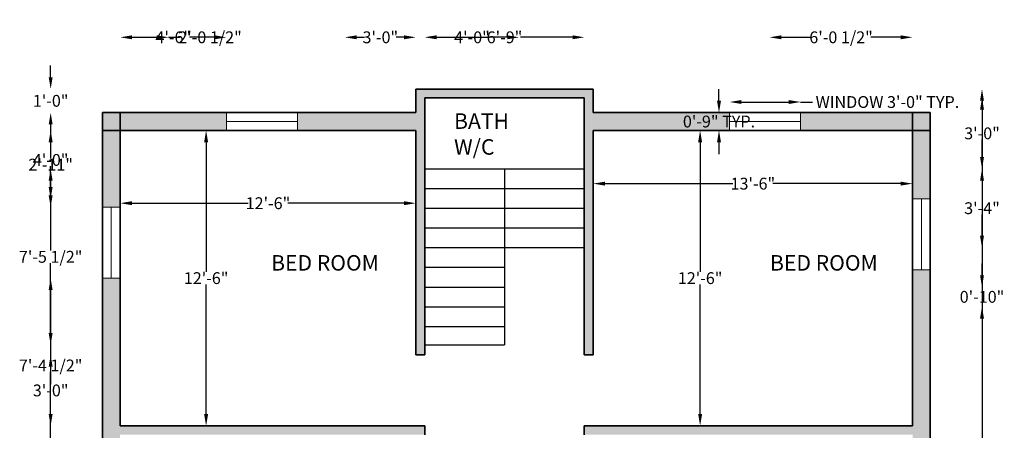
# Model space of a CAD drawing. Units: inches. Extents: x 759 to 1283, y 452 to 1038.
# Tile 3 of 3: x 780 to 1279, y 830 to 1038. Entities that reach past the tile are written whole.
import ezdxf

# ---------------------------------------------------------------- set-up
doc = ezdxf.new("R2010")
doc.units = ezdxf.units.IN
for name, color, linetype, lineweight in [('A-AREA-IDEN', 1, 'Continuous', 25), ('A-COLS', 7, 'Continuous', 35), ('A-COLS-PATT', 7, 'Continuous', 13), ('DIM', 2, 'Continuous', 18), ('STAIR', 7, 'Continuous', 25), ('WALL', 7, 'Continuous', 35), ('WINDOWS', 4, 'Continuous', 18)]:
    doc.layers.add(name, color=color, linetype=linetype, lineweight=lineweight)
doc.layers.add('A-WALL-PATT', color=67, linetype='Continuous', lineweight=13, true_color=0x727430)
doc.styles.get("Standard").update_dxf_attribs({"font": 'arial.ttf'})
doc.dimstyles.get("Standard").update_dxf_attribs({"dimtxt": 6, "dimasz": 6, "dimexe": 0.18, "dimexo": 0.0625, "dimgap": 0.09, "dimtad": 0, "dimtih": 1, "dimtoh": 1, "dimdec": 4, "dimzin": 0, "dimdsep": 46, "dimlunit": 4, "dimtxsty": 'Standard', "dimcen": 0.09, "dimse1": 1, "dimse2": 1, "dimadec": 0, "dimazin": 0, "dimtfac": 1, "dimtdec": 4, "dimtofl": 0, "dimtmove": 0, "dimatfit": 3, "dimfxl": 1, "dimtolj": 1, "dimtzin": 0, "dimarcsym": 0})

# ---------------------------------------------------------------- blocks, each defined once
blk = doc.blocks.new('*D1')
at = {"layer": 'Defpoints', "color": 0, "transparency": 16777216}
for p in [(830.47, 981.81), (980.47, 981.81), (980.47, 944.84)]:
    blk.add_point(p, dxfattribs=at)
at = {"layer": 'DIM', "color": 0, "lineweight": -2, "transparency": 16777216}
for p, q in [((836.47, 944.84), (895.35, 944.84)), ((974.47, 944.84), (915.58, 944.84))]:
    blk.add_line(p, q, dxfattribs=at)
at = {"layer": 'DIM', "color": 0, "transparency": 16777216}
for points in [[(836.47, 945.84), (836.47, 943.84), (830.47, 944.84)], [(974.47, 945.84), (974.47, 943.84), (980.47, 944.84)]]:
    blk.add_solid(points, dxfattribs=at)
at = {"layer": 'DIM', "color": 0, "transparency": 16777216, "insert": (905.47, 944.84), "char_height": 6, "attachment_point": 5}
blk.add_mtext('\\A1;12\'-6"', dxfattribs=at)
blk = doc.blocks.new('*D2')
at = {"layer": 'Defpoints', "color": 0, "transparency": 16777216}
for p in [(830.47, 981.81), (830.47, 831.81), (874.09, 831.81)]:
    blk.add_point(p, dxfattribs=at)
at = {"layer": 'DIM', "color": 0, "lineweight": -2, "transparency": 16777216}
for p, q in [((874.09, 975.81), (874.09, 909.96)), ((874.09, 837.81), (874.09, 903.65))]:
    blk.add_line(p, q, dxfattribs=at)
at = {"layer": 'DIM', "color": 0, "transparency": 16777216}
for points in [[(873.09, 975.81), (875.09, 975.81), (874.09, 981.81)], [(873.09, 837.81), (875.09, 837.81), (874.09, 831.81)]]:
    blk.add_solid(points, dxfattribs=at)
at = {"layer": 'DIM', "color": 0, "transparency": 16777216, "insert": (874.09, 906.81), "char_height": 6, "attachment_point": 5}
blk.add_mtext('\\A1;12\'-6"', dxfattribs=at)
blk = doc.blocks.new('*D3')
at = {"layer": 'Defpoints', "color": 0, "transparency": 16777216}
for p in [(1070.47, 981.81), (1232.47, 981.81), (1232.47, 954.77)]:
    blk.add_point(p, dxfattribs=at)
at = {"layer": 'DIM', "color": 0, "lineweight": -2, "transparency": 16777216}
for p, q in [((1076.47, 954.77), (1141.35, 954.77)), ((1226.47, 954.77), (1161.58, 954.77))]:
    blk.add_line(p, q, dxfattribs=at)
at = {"layer": 'DIM', "color": 0, "transparency": 16777216}
for points in [[(1076.47, 955.77), (1076.47, 953.77), (1070.47, 954.77)], [(1226.47, 955.77), (1226.47, 953.77), (1232.47, 954.77)]]:
    blk.add_solid(points, dxfattribs=at)
at = {"layer": 'DIM', "color": 0, "transparency": 16777216, "insert": (1151.47, 954.77), "char_height": 6, "attachment_point": 5}
blk.add_mtext('\\A1;13\'-6"', dxfattribs=at)
blk = doc.blocks.new('*D4')
at = {"layer": 'Defpoints', "color": 0, "transparency": 16777216}
for p in [(1232.47, 981.81), (1124.71, 831.81), (1232.47, 831.81)]:
    blk.add_point(p, dxfattribs=at)
at = {"layer": 'DIM', "color": 0, "lineweight": -2, "transparency": 16777216}
for p, q in [((1124.71, 975.81), (1124.71, 909.96)), ((1124.71, 837.81), (1124.71, 903.65))]:
    blk.add_line(p, q, dxfattribs=at)
at = {"layer": 'DIM', "color": 0, "transparency": 16777216}
for points in [[(1123.71, 975.81), (1125.71, 975.81), (1124.71, 981.81)], [(1123.71, 837.81), (1125.71, 837.81), (1124.71, 831.81)]]:
    blk.add_solid(points, dxfattribs=at)
at = {"layer": 'DIM', "color": 0, "transparency": 16777216, "insert": (1124.71, 906.81), "char_height": 6, "attachment_point": 5}
blk.add_mtext('\\A1;12\'-6"', dxfattribs=at)
blk = doc.blocks.new('WIN-36IN')
for p, q in [((0, 0), (0, 9)), ((0, 9), (36, 9)), ((36, 9), (36, 0)), ((0, 4.5), (36, 4.5)), ((36, 0), (0, 0))]:
    blk.add_line(p, q)
blk = doc.blocks.new('COL-9X9IN')
for p, q in [((0, 0), (0, 9)), ((0, 9), (9, 9)), ((9, 9), (9, 0)), ((9, 0), (0, 0))]:
    blk.add_line(p, q)
blk = doc.blocks.new('*D19')
at = {"layer": 'Defpoints', "color": 0, "transparency": 16777216}
for p in [(1175.68, 996.21), (1139.68, 990.81), (1175.68, 990.81)]:
    blk.add_point(p, dxfattribs=at)
at = {"layer": 'DIM', "color": 0, "lineweight": -2, "transparency": 16777216}
for p, q in [((1145.68, 996.21), (1169.68, 996.21)), ((1175.68, 996.21), (1181.68, 996.21))]:
    blk.add_line(p, q, dxfattribs=at)
at = {"layer": 'DIM', "color": 0, "transparency": 16777216}
for points in [[(1145.68, 997.21), (1145.68, 995.21), (1139.68, 996.21)], [(1169.68, 997.21), (1169.68, 995.21), (1175.68, 996.21)]]:
    blk.add_solid(points, dxfattribs=at)
at = {"layer": 'DIM', "color": 0, "transparency": 16777216, "insert": (1219.73, 996.21), "char_height": 6, "attachment_point": 5}
blk.add_mtext('\\A1;WINDOW 3\'-0" TYP.', dxfattribs=at)
blk = doc.blocks.new('*D20')
at = {"layer": 'Defpoints', "color": 0, "transparency": 16777216}
for p in [(1134.28, 990.81), (1139.68, 990.81), (1139.68, 981.81)]:
    blk.add_point(p, dxfattribs=at)
at = {"layer": 'DIM', "color": 0, "lineweight": -2, "transparency": 16777216}
for p, q in [((1134.28, 996.81), (1134.28, 1002.81)), ((1134.28, 975.81), (1134.28, 969.81))]:
    blk.add_line(p, q, dxfattribs=at)
at = {"layer": 'DIM', "color": 0, "transparency": 16777216}
for points in [[(1133.28, 996.81), (1135.28, 996.81), (1134.28, 990.81)], [(1133.28, 975.81), (1135.28, 975.81), (1134.28, 981.81)]]:
    blk.add_solid(points, dxfattribs=at)
at = {"layer": 'DIM', "color": 0, "transparency": 16777216, "insert": (1134.28, 986.31), "char_height": 6, "attachment_point": 5}
blk.add_mtext('\\A1;0\'-9" TYP.', dxfattribs=at)
blk = doc.blocks.new('*D24')
at = {"layer": 'Defpoints', "color": 0, "transparency": 16777216}
for p in [(1070.47, 1002.81), (1267.72, 1002.81), (1032.97, 486.81)]:
    blk.add_point(p, dxfattribs=at)
at = {"layer": 'DIM', "color": 0, "lineweight": -2, "transparency": 16777216}
for p, q in [((1267.72, 996.81), (1267.72, 747.96)), ((1267.72, 492.81), (1267.72, 741.65))]:
    blk.add_line(p, q, dxfattribs=at)
at = {"layer": 'DIM', "color": 0, "transparency": 16777216}
for points in [[(1266.72, 996.81), (1268.72, 996.81), (1267.72, 1002.81)], [(1266.72, 492.81), (1268.72, 492.81), (1267.72, 486.81)]]:
    blk.add_solid(points, dxfattribs=at)
at = {"layer": 'DIM', "color": 0, "transparency": 16777216, "insert": (1267.72, 744.81), "char_height": 6, "attachment_point": 5}
blk.add_mtext('\\A1;43\'-0"', dxfattribs=at)
blk = doc.blocks.new('*D25')
at = {"layer": 'Defpoints', "color": 0, "transparency": 16777216}
for p in [(1065.97, 1029.06), (984.97, 998.31), (1065.97, 998.31)]:
    blk.add_point(p, dxfattribs=at)
at = {"layer": 'DIM', "color": 0, "lineweight": -2, "transparency": 16777216}
for p, q in [((990.97, 1029.06), (1017.39, 1029.06)), ((1059.97, 1029.06), (1033.55, 1029.06))]:
    blk.add_line(p, q, dxfattribs=at)
at = {"layer": 'DIM', "color": 0, "transparency": 16777216}
for points in [[(990.97, 1030.06), (990.97, 1028.06), (984.97, 1029.06)], [(1059.97, 1030.06), (1059.97, 1028.06), (1065.97, 1029.06)]]:
    blk.add_solid(points, dxfattribs=at)
at = {"layer": 'DIM', "color": 0, "transparency": 16777216, "insert": (1025.47, 1029.06), "char_height": 6, "attachment_point": 5}
blk.add_mtext('\\A1;6\'-9"', dxfattribs=at)
blk = doc.blocks.new('*D26')
at = {"layer": 'Defpoints', "color": 0, "transparency": 16777216}
for p in [(795.216986, 1002.80698), (980.466986, 1002.80698), (980.466986, 990.80698)]:
    blk.add_point(p, dxfattribs=at)
at = {"layer": 'DIM', "color": 0, "lineweight": -2, "transparency": 16777216}
for p, q in [((795.216986, 1008.80698), (795.216986, 1014.80698)), ((795.216986, 984.80698), (795.216986, 978.80698))]:
    blk.add_line(p, q, dxfattribs=at)
at = {"layer": 'DIM', "color": 0, "transparency": 16777216}
for points in [[(794.216986, 1008.80698), (796.216986, 1008.80698), (795.216986, 1002.80698)], [(794.216986, 984.80698), (796.216986, 984.80698), (795.216986, 990.80698)]]:
    blk.add_solid(points, dxfattribs=at)
at = {"layer": 'DIM', "color": 0, "transparency": 16777216, "insert": (795.216986, 996.80698), "char_height": 6, "attachment_point": 5}
blk.add_mtext('\\A1;1\'-0"', dxfattribs=at)
blk = doc.blocks.new('*D27')
at = {"layer": 'Defpoints', "color": 0, "transparency": 16777216}
for p in [(1032.97, 1029.06), (984.97, 510.81), (1032.97, 510.81)]:
    blk.add_point(p, dxfattribs=at)
at = {"layer": 'DIM', "color": 0, "lineweight": -2, "transparency": 16777216}
for p, q in [((990.97, 1029.06), (1000.78, 1029.06)), ((1026.97, 1029.06), (1017.15, 1029.06))]:
    blk.add_line(p, q, dxfattribs=at)
at = {"layer": 'DIM', "color": 0, "transparency": 16777216}
for points in [[(990.97, 1030.06), (990.97, 1028.06), (984.97, 1029.06)], [(1026.97, 1030.06), (1026.97, 1028.06), (1032.97, 1029.06)]]:
    blk.add_solid(points, dxfattribs=at)
at = {"layer": 'DIM', "color": 0, "transparency": 16777216, "insert": (1008.97, 1029.06), "char_height": 6, "attachment_point": 5}
blk.add_mtext('\\A1;4\'-0"', dxfattribs=at)
blk = doc.blocks.new('*D29')
at = {"layer": 'Defpoints', "color": 0, "transparency": 16777216}
for p in [(830.47, 981.81), (884.41, 981.81), (884.41, 460.56)]:
    blk.add_point(p, dxfattribs=at)
at = {"layer": 'DIM', "color": 0, "lineweight": -2, "transparency": 16777216}
for p, q in [((836.47, 460.56), (849.25, 460.56)), ((878.41, 460.56), (865.62, 460.56))]:
    blk.add_line(p, q, dxfattribs=at)
at = {"layer": 'DIM', "color": 0, "transparency": 16777216}
for points in [[(836.47, 461.56), (836.47, 459.56), (830.47, 460.56)], [(878.41, 461.56), (878.41, 459.56), (884.41, 460.56)]]:
    blk.add_solid(points, dxfattribs=at)
at = {"layer": 'DIM', "color": 0, "transparency": 16777216, "insert": (857.44, 460.56), "char_height": 6, "attachment_point": 5}
blk.add_mtext('\\A1;4\'-6"', dxfattribs=at)
blk = doc.blocks.new('*D30')
at = {"layer": 'Defpoints', "color": 0, "transparency": 16777216}
for p in [(1175.68, 981.81), (1232.47, 981.81), (1232.47, 460.56)]:
    blk.add_point(p, dxfattribs=at)
at = {"layer": 'DIM', "color": 0, "lineweight": -2, "transparency": 16777216}
for p, q in [((1181.68, 460.56), (1195.89, 460.56)), ((1226.47, 460.56), (1212.26, 460.56))]:
    blk.add_line(p, q, dxfattribs=at)
at = {"layer": 'DIM', "color": 0, "transparency": 16777216}
for points in [[(1181.68, 461.56), (1181.68, 459.56), (1175.68, 460.56)], [(1226.47, 461.56), (1226.47, 459.56), (1232.47, 460.56)]]:
    blk.add_solid(points, dxfattribs=at)
at = {"layer": 'DIM', "color": 0, "transparency": 16777216, "insert": (1204.07, 460.56), "char_height": 6, "attachment_point": 5}
blk.add_mtext('\\A1;4\'-9"', dxfattribs=at)
blk = doc.blocks.new('*D31')
at = {"layer": 'Defpoints', "color": 0, "transparency": 16777216}
for p in [(884.41, 1029.06), (830.47, 519.81), (884.41, 519.81)]:
    blk.add_point(p, dxfattribs=at)
at = {"layer": 'DIM', "color": 0, "lineweight": -2, "transparency": 16777216}
for p, q in [((836.47, 1029.06), (849.25, 1029.06)), ((878.41, 1029.06), (865.62, 1029.06))]:
    blk.add_line(p, q, dxfattribs=at)
at = {"layer": 'DIM', "color": 0, "transparency": 16777216}
for points in [[(836.47, 1030.06), (836.47, 1028.06), (830.47, 1029.06)], [(878.41, 1030.06), (878.41, 1028.06), (884.41, 1029.06)]]:
    blk.add_solid(points, dxfattribs=at)
at = {"layer": 'DIM', "color": 0, "transparency": 16777216, "insert": (857.44, 1029.06), "char_height": 6, "attachment_point": 5}
blk.add_mtext('\\A1;4\'-6"', dxfattribs=at)
blk = doc.blocks.new('*D32')
at = {"layer": 'Defpoints', "color": 0, "transparency": 16777216}
for p in [(1232.47, 1029.06), (1159.97, 519.81), (1232.47, 519.81)]:
    blk.add_point(p, dxfattribs=at)
at = {"layer": 'DIM', "color": 0, "lineweight": -2, "transparency": 16777216}
for p, q in [((1165.97, 1029.06), (1181.15, 1029.06)), ((1226.47, 1029.06), (1211.29, 1029.06))]:
    blk.add_line(p, q, dxfattribs=at)
at = {"layer": 'DIM', "color": 0, "transparency": 16777216}
for points in [[(1165.97, 1030.06), (1165.97, 1028.06), (1159.97, 1029.06)], [(1226.47, 1030.06), (1226.47, 1028.06), (1232.47, 1029.06)]]:
    blk.add_solid(points, dxfattribs=at)
at = {"layer": 'DIM', "color": 0, "transparency": 16777216, "insert": (1196.22, 1029.06), "char_height": 6, "attachment_point": 5}
blk.add_mtext('\\A1;6\'-0 1/2"', dxfattribs=at)
blk = doc.blocks.new('*D33')
at = {"layer": 'Defpoints', "color": 0, "transparency": 16777216}
for p in [(821.47, 990.81), (795.22, 942.81), (821.47, 942.81)]:
    blk.add_point(p, dxfattribs=at)
at = {"layer": 'DIM', "color": 0, "lineweight": -2, "transparency": 16777216}
for p, q in [((795.22, 984.81), (795.22, 969.96)), ((795.22, 948.81), (795.22, 963.65))]:
    blk.add_line(p, q, dxfattribs=at)
at = {"layer": 'DIM', "color": 0, "transparency": 16777216}
for points in [[(794.22, 984.81), (796.22, 984.81), (795.22, 990.81)], [(794.22, 948.81), (796.22, 948.81), (795.22, 942.81)]]:
    blk.add_solid(points, dxfattribs=at)
at = {"layer": 'DIM', "color": 0, "transparency": 16777216, "insert": (795.22, 966.81), "char_height": 6, "attachment_point": 5}
blk.add_mtext('\\A1;4\'-0"', dxfattribs=at)
blk = doc.blocks.new('*D34')
at = {"layer": 'Defpoints', "color": 0, "transparency": 16777216}
for p in [(821.47, 906.81), (795.22, 818.14), (821.47, 818.14)]:
    blk.add_point(p, dxfattribs=at)
at = {"layer": 'DIM', "color": 0, "lineweight": -2, "transparency": 16777216}
for p, q in [((795.22, 900.81), (795.22, 865.67)), ((795.22, 824.14), (795.22, 859.28))]:
    blk.add_line(p, q, dxfattribs=at)
at = {"layer": 'DIM', "color": 0, "transparency": 16777216}
for points in [[(794.22, 900.81), (796.22, 900.81), (795.22, 906.81)], [(794.22, 824.14), (796.22, 824.14), (795.22, 818.14)]]:
    blk.add_solid(points, dxfattribs=at)
at = {"layer": 'DIM', "color": 0, "transparency": 16777216, "insert": (795.22, 862.47), "char_height": 6, "attachment_point": 5}
blk.add_mtext('\\A1;7\'-4 1/2"', dxfattribs=at)
blk = doc.blocks.new('*D37')
at = {"layer": 'Defpoints', "color": 0, "transparency": 16777216}
for p in [(1232.47, 981.81), (795.22, 947.03), (1232.47, 947.03)]:
    blk.add_point(p, dxfattribs=at)
at = {"layer": 'DIM', "color": 0, "lineweight": -2, "transparency": 16777216}
for p, q in [((795.22, 975.81), (795.22, 967.52)), ((795.22, 953.03), (795.22, 961.32))]:
    blk.add_line(p, q, dxfattribs=at)
at = {"layer": 'DIM', "color": 0, "transparency": 16777216}
for points in [[(794.22, 975.81), (796.22, 975.81), (795.22, 981.81)], [(794.22, 953.03), (796.22, 953.03), (795.22, 947.03)]]:
    blk.add_solid(points, dxfattribs=at)
at = {"layer": 'DIM', "color": 0, "transparency": 16777216, "insert": (795.22, 964.42), "char_height": 6, "attachment_point": 5}
blk.add_mtext('\\A1;2\'-11"', dxfattribs=at)
blk = doc.blocks.new('*D40')
at = {"layer": 'Defpoints', "color": 0, "transparency": 16777216}
for p in [(984.97, 998.31), (984.97, 962.31), (1267.72, 962.31)]:
    blk.add_point(p, dxfattribs=at)
at = {"layer": 'DIM', "color": 0, "lineweight": -2, "transparency": 16777216}
for p, q in [((1267.72, 992.31), (1267.72, 983.46)), ((1267.72, 968.31), (1267.72, 977.15))]:
    blk.add_line(p, q, dxfattribs=at)
at = {"layer": 'DIM', "color": 0, "transparency": 16777216}
for points in [[(1266.72, 992.31), (1268.72, 992.31), (1267.72, 998.31)], [(1266.72, 968.31), (1268.72, 968.31), (1267.72, 962.31)]]:
    blk.add_solid(points, dxfattribs=at)
at = {"layer": 'DIM', "color": 0, "transparency": 16777216, "insert": (1267.72, 980.31), "char_height": 6, "attachment_point": 5}
blk.add_mtext('\\A1;3\'-0"', dxfattribs=at)
blk = doc.blocks.new('*D41')
at = {"layer": 'Defpoints', "color": 0, "transparency": 16777216}
for p in [(984.966986, 872.954802), (1025.466986, 872.954802), (1025.466986, 460.55698)]:
    blk.add_point(p, dxfattribs=at)
at = {"layer": 'DIM', "color": 0, "lineweight": -2, "transparency": 16777216}
for p, q in [((978.966986, 460.55698), (972.966986, 460.55698)), ((1031.466986, 460.55698), (1037.466986, 460.55698))]:
    blk.add_line(p, q, dxfattribs=at)
at = {"layer": 'DIM', "color": 0, "transparency": 16777216}
for points in [[(978.966986, 461.55698), (978.966986, 459.55698), (984.966986, 460.55698)], [(1031.466986, 461.55698), (1031.466986, 459.55698), (1025.466986, 460.55698)]]:
    blk.add_solid(points, dxfattribs=at)
at = {"layer": 'DIM', "color": 0, "transparency": 16777216, "insert": (1005.216986, 460.55698), "char_height": 6, "attachment_point": 5}
blk.add_mtext('\\A1;3\'-4 1/2"', dxfattribs=at)
blk = doc.blocks.new('*D42')
at = {"layer": 'Defpoints', "color": 0, "transparency": 16777216}
for p in [(984.97, 867.81), (795.22, 831.81), (984.97, 831.81)]:
    blk.add_point(p, dxfattribs=at)
at = {"layer": 'DIM', "color": 0, "lineweight": -2, "transparency": 16777216}
for p, q in [((795.22, 861.81), (795.22, 852.96)), ((795.22, 837.81), (795.22, 846.65))]:
    blk.add_line(p, q, dxfattribs=at)
at = {"layer": 'DIM', "color": 0, "transparency": 16777216}
for points in [[(794.22, 861.81), (796.22, 861.81), (795.22, 867.81)], [(794.22, 837.81), (796.22, 837.81), (795.22, 831.81)]]:
    blk.add_solid(points, dxfattribs=at)
at = {"layer": 'DIM', "color": 0, "transparency": 16777216, "insert": (795.22, 849.81), "char_height": 6, "attachment_point": 5}
blk.add_mtext('\\A1;3\'-0"', dxfattribs=at)
blk = doc.blocks.new('*D46')
at = {"layer": 'Defpoints', "color": 0, "transparency": 16777216}
for p in [(980.47, 1029.06), (944.47, 660.31), (980.47, 660.31)]:
    blk.add_point(p, dxfattribs=at)
at = {"layer": 'DIM', "color": 0, "lineweight": -2, "transparency": 16777216}
for p, q in [((950.47, 1029.06), (954.4, 1029.06)), ((974.47, 1029.06), (970.53, 1029.06))]:
    blk.add_line(p, q, dxfattribs=at)
at = {"layer": 'DIM', "color": 0, "transparency": 16777216}
for points in [[(950.47, 1030.06), (950.47, 1028.06), (944.47, 1029.06)], [(974.47, 1030.06), (974.47, 1028.06), (980.47, 1029.06)]]:
    blk.add_solid(points, dxfattribs=at)
at = {"layer": 'DIM', "color": 0, "transparency": 16777216, "insert": (962.47, 1029.06), "char_height": 6, "attachment_point": 5}
blk.add_mtext('\\A1;3\'-0"', dxfattribs=at)
blk = doc.blocks.new('*D47')
at = {"layer": 'Defpoints', "color": 0, "transparency": 16777216}
for p in [(795.22, 962.31), (984.97, 962.31), (984.97, 872.95)]:
    blk.add_point(p, dxfattribs=at)
at = {"layer": 'DIM', "color": 0, "lineweight": -2, "transparency": 16777216}
for p, q in [((795.22, 956.31), (795.22, 920.82)), ((795.22, 878.95), (795.22, 914.44))]:
    blk.add_line(p, q, dxfattribs=at)
at = {"layer": 'DIM', "color": 0, "transparency": 16777216}
for points in [[(794.22, 956.31), (796.22, 956.31), (795.22, 962.31)], [(794.22, 878.95), (796.22, 878.95), (795.22, 872.95)]]:
    blk.add_solid(points, dxfattribs=at)
at = {"layer": 'DIM', "color": 0, "transparency": 16777216, "insert": (795.22, 917.63), "char_height": 6, "attachment_point": 5}
blk.add_mtext('\\A1;7\'-5 1/2"', dxfattribs=at)
blk = doc.blocks.new('*D48')
at = {"layer": 'Defpoints', "color": 0, "transparency": 16777216}
for p in [(1025.466986, 902.30698), (1267.716986, 902.30698), (1025.466986, 892.30698)]:
    blk.add_point(p, dxfattribs=at)
at = {"layer": 'DIM', "color": 0, "lineweight": -2, "transparency": 16777216}
for p, q in [((1267.716986, 908.30698), (1267.716986, 914.30698)), ((1267.716986, 886.30698), (1267.716986, 880.30698))]:
    blk.add_line(p, q, dxfattribs=at)
at = {"layer": 'DIM', "color": 0, "transparency": 16777216}
for points in [[(1266.716986, 908.30698), (1268.716986, 908.30698), (1267.716986, 902.30698)], [(1266.716986, 886.30698), (1268.716986, 886.30698), (1267.716986, 892.30698)]]:
    blk.add_solid(points, dxfattribs=at)
at = {"layer": 'DIM', "color": 0, "transparency": 16777216, "insert": (1267.716986, 897.30698), "char_height": 6, "attachment_point": 5}
blk.add_mtext('\\A1;0\'-10"', dxfattribs=at)
blk = doc.blocks.new('*D49')
at = {"layer": 'Defpoints', "color": 0, "transparency": 16777216}
for p in [(1065.97, 962.31), (1267.72, 962.31), (1065.97, 922.31)]:
    blk.add_point(p, dxfattribs=at)
at = {"layer": 'DIM', "color": 0, "lineweight": -2, "transparency": 16777216}
for p, q in [((1267.72, 956.31), (1267.72, 945.46)), ((1267.72, 928.31), (1267.72, 939.15))]:
    blk.add_line(p, q, dxfattribs=at)
at = {"layer": 'DIM', "color": 0, "transparency": 16777216}
for points in [[(1266.72, 956.31), (1268.72, 956.31), (1267.72, 962.31)], [(1266.72, 928.31), (1268.72, 928.31), (1267.72, 922.31)]]:
    blk.add_solid(points, dxfattribs=at)
at = {"layer": 'DIM', "color": 0, "transparency": 16777216, "insert": (1267.72, 942.31), "char_height": 6, "attachment_point": 5}
blk.add_mtext('\\A1;3\'-4"', dxfattribs=at)
blk = doc.blocks.new('*D50')
at = {"layer": 'Defpoints', "color": 0, "transparency": 16777216}
for p in [(854.96, 1029.06), (830.47, 664.81), (854.96, 664.81)]:
    blk.add_point(p, dxfattribs=at)
at = {"layer": 'DIM', "color": 0, "lineweight": -2, "transparency": 16777216}
for p, q in [((836.47, 1029.06), (848.96, 1029.06)), ((854.96, 1029.06), (860.96, 1029.06))]:
    blk.add_line(p, q, dxfattribs=at)
at = {"layer": 'DIM', "color": 0, "transparency": 16777216}
for points in [[(836.47, 1030.06), (836.47, 1028.06), (830.47, 1029.06)], [(848.96, 1030.06), (848.96, 1028.06), (854.96, 1029.06)]]:
    blk.add_solid(points, dxfattribs=at)
at = {"layer": 'DIM', "color": 0, "transparency": 16777216, "insert": (876.07, 1029.06), "char_height": 6, "attachment_point": 5}
blk.add_mtext('\\A1;2\'-0 1/2"', dxfattribs=at)

msp = doc.modelspace()

# ---------------------------------------------------------------- hatches: boundary and pattern name
at = {"layer": 'A-COLS-PATT'}
h = msp.add_hatch(color=256, dxfattribs=at)
h.dxf.hatch_style = 1
h.paths.add_polyline_path([(1241.46699, 990.80698), (1232.46699, 990.80698), (1232.46699, 981.80698), (1241.46699, 981.80698)])
h.paths.add_polyline_path([(830.46699, 990.80698), (821.46699, 990.80698), (821.46699, 981.80698), (830.46699, 981.80698)])
h.paths.add_polyline_path([(830.46699, 519.80698), (821.46699, 519.80698), (821.46699, 510.80698), (830.46699, 510.80698)])
h.paths.add_polyline_path([(1241.46699, 519.80698), (1232.46699, 519.80698), (1232.46699, 510.80698), (1241.46699, 510.80698)])
at = {"layer": 'A-WALL-PATT'}
h = msp.add_hatch(color=256, dxfattribs=at)
h.dxf.hatch_style = 1
h.paths.add_polyline_path([(1232.46699, 519.80698), (1159.97269, 519.80698), (1159.97269, 510.80698), (1232.46699, 510.80698)])
h.paths.add_polyline_path([(1241.46699, 580.365), (1232.46699, 580.365), (1232.46699, 519.80698), (1241.46699, 519.80698)])
h.paths.add_polyline_path([(1123.97269, 519.80698), (1032.96699, 519.80698), (1032.96699, 510.80698), (1123.97269, 510.80698)])
h.paths.add_polyline_path([(984.96699, 519.80698), (984.96699, 664.80698), (980.46699, 664.80698), (980.46699, 660.30698), (980.46699, 519.80698), (920.40841, 519.80698), (920.40841, 510.80698), (984.96699, 510.80698)])
h.paths.add_polyline_path([(884.40841, 519.80698), (830.46699, 519.80698), (830.46699, 510.80698), (884.40841, 510.80698)])
h.paths.add_polyline_path([(830.46699, 590.05698), (821.46699, 590.05698), (821.46699, 519.80698), (830.46699, 519.80698)])
h.paths.add_polyline_path([(830.46699, 660.30698), (944.46699, 660.30698), (944.46699, 664.80698), (830.46699, 664.80698), (830.46699, 691.13164), (821.46699, 691.13164), (821.46699, 626.05698), (830.46699, 626.05698)])
h.paths.add_polyline_path([(830.46699, 767.80698), (914.46699, 767.80698), (914.46699, 726.32345), (918.96699, 726.32345), (918.96699, 775.80521), (918.96699, 790.30698), (914.46699, 790.30698), (914.46699, 772.30698), (830.46699, 772.30698), (830.46699, 782.14186), (821.46699, 782.14186), (821.46699, 727.13164), (830.46699, 727.13164)])
h.paths.add_polyline_path([(830.46699, 906.80698), (821.46699, 906.80698), (821.46699, 818.14186), (830.46699, 818.14186), (830.46699, 827.30698), (984.96699, 827.30698), (984.96699, 831.80698), (980.46699, 831.80698), (830.46699, 831.80698)])
h.paths.add_polyline_path([(830.46699, 981.80698), (821.46699, 981.80698), (821.46699, 942.80698), (830.46699, 942.80698)])
h.paths.add_polyline_path([(884.40841, 990.80698), (830.46699, 990.80698), (830.46699, 981.80698), (884.40841, 981.80698)])
h.paths.add_polyline_path([(984.96699, 998.30698), (1065.96699, 998.30698), (1065.96699, 981.80698), (1065.96699, 867.80698), (1070.46699, 867.80698), (1070.46699, 981.80698), (1139.68016, 981.80698), (1139.68016, 990.80698), (1070.46699, 990.80698), (1070.46699, 1002.80698), (980.46699, 1002.80698), (980.46699, 990.80698), (920.40841, 990.80698), (920.40841, 981.80698), (980.46699, 981.80698), (980.46699, 867.80698), (984.96699, 867.80698), (984.96699, 981.80698)])
h.paths.add_polyline_path([(1232.46699, 990.80698), (1175.68016, 990.80698), (1175.68016, 981.80698), (1232.46699, 981.80698)])
h.paths.add_polyline_path([(1241.46699, 981.80698), (1232.46699, 981.80698), (1232.46699, 947.03418), (1241.46699, 947.03418)])
h.paths.add_polyline_path([(1241.46699, 911.03418), (1232.46699, 911.03418), (1232.46699, 831.80698), (1070.46699, 831.80698), (1065.96699, 831.80698), (1065.96699, 827.30698), (1070.46699, 827.30698), (1232.46699, 827.30698), (1232.46699, 770.87725), (1241.46699, 770.87725)])
h.paths.add_polyline_path([(1241.46699, 734.87725), (1232.46699, 734.87725), (1232.46699, 671.30698), (1070.46699, 671.30698), (1070.46699, 666.80698), (1232.46699, 666.80698), (1232.46699, 616.365), (1241.46699, 616.365)])
h.paths.add_polyline_path([(1070.46699, 791.30698), (1065.96699, 791.30698), (1065.96699, 666.80698), (1070.46699, 666.80698)])

# ---------------------------------------------------------------- linework, layer by layer
at = {"layer": 'STAIR'}
for p, q in [((984.96699, 962.30698), (1065.96699, 962.30698)), ((1025.46699, 962.30698), (1025.46699, 872.9548)), ((984.96699, 952.30698), (1065.96699, 952.30698)), ((984.96699, 942.30698), (1065.96699, 942.30698)), ((984.96699, 932.30698), (1065.96699, 932.30698)), ((984.96699, 922.30698), (1065.96699, 922.30698)), ((984.96699, 912.30698), (1025.46699, 912.30698)), ((984.96699, 902.30698), (1025.46699, 902.30698)), ((984.96699, 892.30698), (1025.46699, 892.30698)), ((984.96699, 882.30698), (1025.46699, 882.30698)), ((984.96699, 872.9548), (1025.46699, 872.9548))]:
    msp.add_line(p, q, dxfattribs=at)
at = {"layer": 'WALL'}
for p, q in [((980.46699, 990.80698), (980.46699, 1002.80698)), ((980.46699, 1002.80698), (1070.46699, 1002.80698)), ((1070.46699, 1002.80698), (1070.46699, 990.80698)), ((984.96699, 981.80698), (984.96699, 998.30698)), ((984.96699, 998.30698), (1065.96699, 998.30698)), ((1065.96699, 981.80698), (1065.96699, 998.30698)), ((821.46699, 990.80698), (821.46699, 510.80698)), ((821.46699, 990.80698), (980.46699, 990.80698)), ((1070.46699, 990.80698), (1241.46699, 990.80698)), ((1241.46699, 990.80698), (1241.46699, 510.80698)), ((830.46699, 981.80698), (830.46699, 831.80698)), ((830.46699, 981.80698), (980.46699, 981.80698)), ((980.46699, 981.80698), (980.46699, 867.80698)), ((984.96699, 981.80698), (984.96699, 867.80698)), ((1065.96699, 981.80698), (1065.96699, 867.80698)), ((1070.46699, 981.80698), (1070.46699, 867.80698)), ((1070.46699, 981.80698), (1232.46699, 981.80698)), ((1232.46699, 981.80698), (1232.46699, 831.80698)), ((980.46699, 867.80698), (984.96699, 867.80698)), ((1065.96699, 867.80698), (1070.46699, 867.80698)), ((830.46699, 831.80698), (980.46699, 831.80698)), ((984.96699, 831.80698), (980.46699, 831.80698)), ((984.96699, 831.80698), (984.96699, 827.30698)), ((1070.46699, 831.80698), (1065.96699, 831.80698)), ((1065.96699, 831.80698), (1065.96699, 827.30698)), ((1070.46699, 831.80698), (1232.46699, 831.80698))]:
    msp.add_line(p, q, dxfattribs=at)

# ---------------------------------------------------------------- block references
at = {"layer": 'A-COLS'}
msp.add_blockref('COL-9X9IN', (821.467, 981.807), dxfattribs=at)
at = {"layer": 'A-COLS', "rotation": 180}
msp.add_blockref('COL-9X9IN', (1241.46697, 990.80696), dxfattribs=at)
at = {"layer": 'WINDOWS'}
for p in [(884.408, 981.807), (1139.67975, 981.807)]:
    msp.add_blockref('WIN-36IN', p, dxfattribs=at)
for p, rotation in [((1232.46701, 947.03459), 270.0000000000004), ((821.46701, 942.80739), 270.0000000000001)]:
    msp.add_blockref('WIN-36IN', p, dxfattribs=dict(at, rotation=rotation))

# ---------------------------------------------------------------- texts
at = {"layer": 'A-AREA-IDEN', "char_height": 7.875, "attachment_point": 1}
for s, insert in [('BATH \\PW/C', (999.87334, 990.46844)), ('BED ROOM', (907.06739, 918.50186)), ('BED ROOM', (1160.16986, 918.50186))]:
    msp.add_mtext_dynamic_manual_height_columns(s, width=120.4934303, gutter_width=39.375, heights=[0], dxfattribs=dict(at, insert=insert))

# ---------------------------------------------------------------- dimensions: what is measured, and where the dimension line sits
at = {"layer": 'DIM'}
for base, p1, p2, override, picture, middle in [((854.96067, 1029.05698), (830.46699, 664.80698), (854.96067, 664.80698), {"dimdec": 1, "dimlfac": 1, "dimrnd": 0, "dimzin": 1, "dimdsep": 46, "dimlunit": 4, "dimfrac": 2}, '*D50', (876.06704, 1029.05698)), ((1232.46699, 1029.05698), (1159.97269, 519.80698), (1232.46699, 519.80698), {"dimdec": 1, "dimlfac": 1, "dimrnd": 0, "dimzin": 1, "dimdsep": 46, "dimlunit": 4, "dimfrac": 2}, '*D32', (1196.21984, 1029.05698)), ((884.40841, 1029.05698), (830.46699, 519.80698), (884.40841, 519.80698), {"dimdec": 1, "dimlfac": 1, "dimrnd": 0, "dimzin": 1, "dimdsep": 46, "dimlunit": 4, "dimfrac": 2}, '*D31', (857.4377, 1029.05698)), ((980.46699, 1029.05698), (944.46699, 660.30698), (980.46699, 660.30698), {"dimdec": 1, "dimlfac": 1, "dimrnd": 0, "dimzin": 1, "dimdsep": 46, "dimlunit": 4, "dimfrac": 2}, '*D46', (962.46699, 1029.05698)), ((1065.96699, 1029.05698), (984.96699, 998.30698), (1065.96699, 998.30698), {"dimdec": 1, "dimlfac": 1, "dimrnd": 0, "dimzin": 1, "dimdsep": 46, "dimlunit": 4, "dimfrac": 2}, '*D25', (1025.46699, 1029.05698)), ((1032.96699, 1029.05698), (984.96699, 510.80698), (1032.96699, 510.80698), {"dimdec": 1, "dimlfac": 1, "dimrnd": 0, "dimzin": 1, "dimdsep": 46, "dimlunit": 4, "dimfrac": 2}, '*D27', (1008.96699, 1029.05698)), ((980.46699, 944.83669), (830.46699, 981.80698), (980.46699, 981.80698), {"dimclrd": 0, "dimclre": 0, "dimclrt": 0}, '*D1', (905.46699, 944.83669)), ((884.40841, 460.55698), (830.46699, 981.80698), (884.40841, 981.80698), {"dimdec": 1, "dimlfac": 1, "dimrnd": 0, "dimzin": 1, "dimdsep": 46, "dimlunit": 4, "dimfrac": 2}, '*D29', (857.4377, 460.55698)), ((1232.46699, 954.76921), (1070.46699, 981.80698), (1232.46699, 981.80698), {"dimclrd": 0, "dimclre": 0, "dimclrt": 0}, '*D3', (1151.46699, 954.76921)), ((1232.46699, 460.55698), (1175.68016, 981.80698), (1232.46699, 981.80698), {"dimdec": 1, "dimlfac": 1, "dimrnd": 0, "dimzin": 1, "dimdsep": 46, "dimlunit": 4, "dimfrac": 2}, '*D30', (1204.07357, 460.55698)), ((1025.46699, 460.55698), (984.96699, 872.9548), (1025.46699, 872.9548), {"dimdec": 1, "dimlfac": 1, "dimrnd": 0, "dimzin": 1, "dimdsep": 46, "dimlunit": 4, "dimfrac": 2}, '*D41', (1005.21699, 460.55698))]:
    dim = msp.add_linear_dim(base=base, p1=p1, p2=p2, dimstyle='Standard', override=override, dxfattribs=at)
    dim.commit()
    dim.dimension.update_dxf_attribs({"geometry": picture, "text_midpoint": middle})
for base, p1, p2, override, picture, middle in [((795.21699, 1002.80698), (980.46699, 990.80698), (980.46699, 1002.80698), {"dimdec": 1, "dimlfac": 1, "dimrnd": 0, "dimzin": 1, "dimdsep": 46, "dimlunit": 4, "dimfrac": 2}, '*D26', (795.21699, 996.80698)), ((1267.71699, 1002.80698), (1032.96699, 486.80698), (1070.46699, 1002.80698), {"dimdec": 1, "dimlfac": 1, "dimrnd": 0, "dimzin": 1, "dimdsep": 46, "dimlunit": 4, "dimfrac": 2}, '*D24', (1267.71699, 744.80698)), ((1267.71699, 962.30698), (984.96699, 998.30698), (984.96699, 962.30698), {"dimdec": 1, "dimlfac": 1, "dimrnd": 0, "dimzin": 1, "dimdsep": 46, "dimlunit": 4, "dimfrac": 2}, '*D40', (1267.71699, 980.30698)), ((795.21699, 942.80698), (821.46699, 990.80698), (821.46699, 942.80698), {"dimdec": 1, "dimlfac": 1, "dimrnd": 0, "dimzin": 1, "dimdsep": 46, "dimlunit": 4, "dimfrac": 2}, '*D33', (795.21699, 966.80698)), ((795.21699, 947.03418), (1232.46699, 981.80698), (1232.46699, 947.03418), {"dimdec": 1, "dimlfac": 1, "dimrnd": 0, "dimzin": 1, "dimdsep": 46, "dimlunit": 4, "dimfrac": 2}, '*D37', (795.21699, 964.42058)), ((874.08786, 831.80698), (830.46699, 981.80698), (830.46699, 831.80698), {"dimclrd": 0, "dimclre": 0, "dimclrt": 0}, '*D2', (874.08786, 906.80698)), ((1124.71207, 831.80698), (1232.46699, 981.80698), (1232.46699, 831.80698), {"dimclrd": 0, "dimclre": 0, "dimclrt": 0}, '*D4', (1124.71207, 906.80698)), ((795.21699, 962.30698), (984.96699, 872.9548), (984.96699, 962.30698), {"dimdec": 1, "dimlfac": 1, "dimrnd": 0, "dimzin": 1, "dimdsep": 46, "dimlunit": 4, "dimfrac": 2}, '*D47', (795.21699, 917.63089)), ((1267.71699, 962.30698), (1065.96699, 922.30698), (1065.96699, 962.30698), {"dimdec": 1, "dimlfac": 1, "dimrnd": 0, "dimzin": 1, "dimdsep": 46, "dimlunit": 4, "dimfrac": 2}, '*D49', (1267.71699, 942.30698)), ((1267.71699, 902.30698), (1025.46699, 892.30698), (1025.46699, 902.30698), {"dimdec": 1, "dimlfac": 1, "dimrnd": 0, "dimzin": 1, "dimdsep": 46, "dimlunit": 4, "dimfrac": 2}, '*D48', (1267.71699, 897.30698)), ((795.21699, 818.14186), (821.46699, 906.80698), (821.46699, 818.14186), {"dimdec": 1, "dimlfac": 1, "dimrnd": 0, "dimzin": 1, "dimdsep": 46, "dimlunit": 4, "dimfrac": 2}, '*D34', (795.21699, 862.47442)), ((795.21699, 831.80698), (984.96699, 867.80698), (984.96699, 831.80698), {"dimdec": 1, "dimlfac": 1, "dimrnd": 0, "dimzin": 1, "dimdsep": 46, "dimlunit": 4, "dimfrac": 2}, '*D42', (795.21699, 849.80698))]:
    dim = msp.add_linear_dim(base=base, p1=p1, p2=p2, angle=90, dimstyle='Standard', override=override, dxfattribs=at)
    dim.commit()
    dim.dimension.update_dxf_attribs({"geometry": picture, "text_midpoint": middle})
dim = msp.add_linear_dim(base=(1175.68016, 996.20698), p1=(1139.68016, 990.80698), p2=(1175.68016, 990.80698), text='WINDOW <> TYP.', dimstyle='Standard', override={"dimdec": 1, "dimlfac": 1, "dimrnd": 0, "dimzin": 1, "dimdsep": 46, "dimlunit": 4, "dimfrac": 2}, dxfattribs=at)
dim.commit()
dim.dimension.update_dxf_attribs({"geometry": '*D19', "text_midpoint": (1219.73264, 996.20698)})
dim = msp.add_linear_dim(base=(1134.28016, 990.80698), p1=(1139.68016, 981.80698), p2=(1139.68016, 990.80698), angle=90, text='<> TYP.', dimstyle='Standard', override={"dimdec": 1, "dimlfac": 1, "dimrnd": 0, "dimzin": 1, "dimdsep": 46, "dimlunit": 4, "dimfrac": 2}, dxfattribs=at)
dim.commit()
dim.dimension.update_dxf_attribs({"geometry": '*D20', "text_midpoint": (1134.28016, 986.30698)})

doc.saveas('drawing.dxf')
